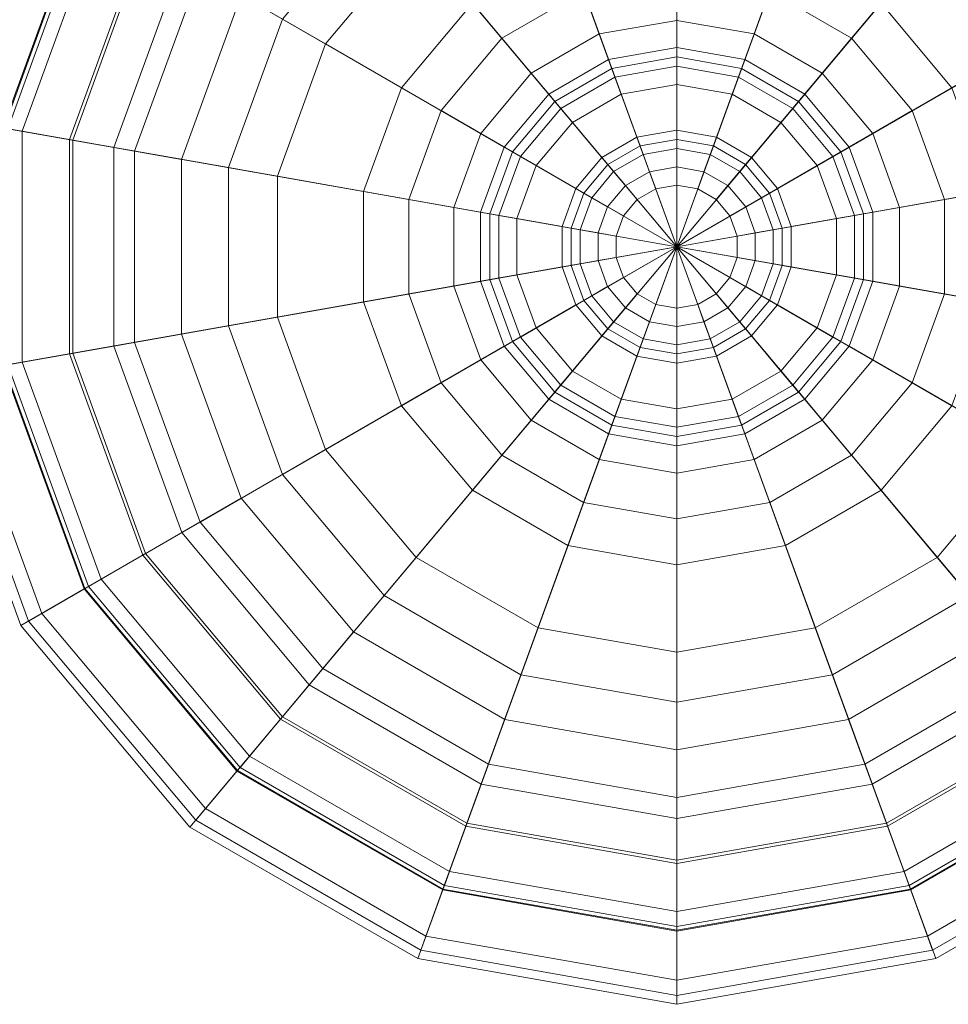
# Model space of a CAD drawing. Units: inches. Extents: x 375 to 1122, y 27 to 1069.
# Tile 48 of 155: x 720.906 to 722.566, y 309.111 to 310.871. Entities that reach past the tile are written whole.
import ezdxf

# ---------------------------------------------------------------- set-up
doc = ezdxf.new("R2010")
doc.units = ezdxf.units.IN
doc.layers.add('Furniture', color=30, linetype='Continuous', lineweight=18)

# ---------------------------------------------------------------- blocks, each defined once
blk = doc.blocks.new('A$C403C54AD')
for points in [[(0.889855, 0.961682, -0.042784), (0.895735, 0.928335, -0.039705), (0.895735, 0.928335, -0.039705), (0.878804, 0.95766, -0.042784)], [(0.901615, 0.961682, -0.042784), (0.895735, 0.928335, -0.039705), (0.895735, 0.928335, -0.039705), (0.889855, 0.961682, -0.042784)], [(0.912666, 0.95766, -0.042784), (0.895735, 0.928335, -0.039705), (0.895735, 0.928335, -0.039705), (0.901615, 0.961682, -0.042784)], [(0.878804, 0.95766, -0.042784), (0.895735, 0.928335, -0.039705), (0.895735, 0.928335, -0.039705), (0.869795, 0.950101, -0.042784)], [(0.921675, 0.950101, -0.042784), (0.895735, 0.928335, -0.039705), (0.895735, 0.928335, -0.039705), (0.912666, 0.95766, -0.042784)], [(0.888627, 0.940645, -0.036278), (0.880436, 0.954832, -0.039553), (0.872296, 0.948002, -0.039553), (0.884846, 0.937471, -0.036278)], [(0.906623, 0.937471, -0.036278), (0.919173, 0.948002, -0.039553), (0.911033, 0.954832, -0.039553), (0.902842, 0.940645, -0.036278)], [(0.869795, 0.950101, -0.042784), (0.895735, 0.928335, -0.039705), (0.895735, 0.928335, -0.039705), (0.863915, 0.939916, -0.042784)], [(0.927555, 0.939916, -0.042784), (0.895735, 0.928335, -0.039705), (0.895735, 0.928335, -0.039705), (0.921675, 0.950101, -0.042784)], [(0.924448, 0.938785, 0.1202), (0.92718, 0.93978, 0.106976), (0.921369, 0.949844, 0.106976), (0.919142, 0.947976, 0.1202)], [(0.924486, 0.938799, -0.039553), (0.927555, 0.939916, -0.042784), (0.921675, 0.950101, -0.042784), (0.919173, 0.948002, -0.039553)], [(0.92718, 0.93978, 0.106976), (0.926546, 0.939549, 0.078734), (0.920852, 0.949411, 0.078734), (0.921369, 0.949844, 0.106976)], [(0.886671, 0.944033, 0.05268), (0.883428, 0.94965, 0.062072), (0.87688, 0.944156, 0.062072), (0.881848, 0.939987, 0.05268)], [(0.909621, 0.939987, 0.05268), (0.914589, 0.944156, 0.062072), (0.908041, 0.94965, 0.062072), (0.904798, 0.944033, 0.05268)], [(0.926546, 0.939549, 0.078734), (0.921505, 0.937714, 0.060725), (0.916743, 0.945962, 0.060725), (0.920852, 0.949411, 0.078734)], [(0.8922, 0.948383, 0.050493), (0.893978, 0.9383, 0.043125), (0.890675, 0.937098, 0.043125), (0.885556, 0.945965, 0.050493)], [(0.89927, 0.948383, 0.050493), (0.897492, 0.9383, 0.043125), (0.893978, 0.9383, 0.043125), (0.8922, 0.948383, 0.050493)], [(0.905913, 0.945965, 0.050493), (0.900794, 0.937098, 0.043125), (0.897492, 0.9383, 0.043125), (0.89927, 0.948383, 0.050493)], [(0.909092, 0.933196, -0.036278), (0.924486, 0.938799, -0.039553), (0.919173, 0.948002, -0.039553), (0.906623, 0.937471, -0.036278)], [(0.919753, 0.937076, 0.129606), (0.924448, 0.938785, 0.1202), (0.919142, 0.947976, 0.1202), (0.915314, 0.944764, 0.129606)], [(0.924281, 0.938725, 0.106759), (0.921641, 0.937764, 0.119395), (0.916854, 0.946056, 0.119395), (0.919006, 0.947862, 0.106759)], [(0.923663, 0.9385, 0.079219), (0.924281, 0.938725, 0.106759), (0.919006, 0.947862, 0.106759), (0.918502, 0.947439, 0.079219)], [(0.918863, 0.936753, 0.062072), (0.923663, 0.9385, 0.079219), (0.918502, 0.947439, 0.079219), (0.914589, 0.944156, 0.062072)], [(0.885556, 0.945965, 0.050493), (0.890675, 0.937098, 0.043125), (0.887983, 0.934839, 0.043125), (0.88014, 0.94142, 0.050493)], [(0.894188, 0.937103, 0.046044), (0.892587, 0.946186, 0.05268), (0.886671, 0.944033, 0.05268), (0.891283, 0.936046, 0.046044)], [(0.897281, 0.937103, 0.046044), (0.898882, 0.946186, 0.05268), (0.892587, 0.946186, 0.05268), (0.894188, 0.937103, 0.046044)], [(0.900187, 0.936046, 0.046044), (0.904798, 0.944033, 0.05268), (0.898882, 0.946186, 0.05268), (0.897281, 0.937103, 0.046044)], [(0.911329, 0.94142, 0.050493), (0.903486, 0.934839, 0.043125), (0.900794, 0.937098, 0.043125), (0.905913, 0.945965, 0.050493)], [(0.921505, 0.937714, 0.060725), (0.914864, 0.935297, 0.050493), (0.911329, 0.94142, 0.050493), (0.916743, 0.945962, 0.060725)], [(0.921641, 0.937764, 0.119395), (0.91686, 0.936024, 0.129606), (0.912956, 0.942785, 0.129606), (0.916854, 0.946056, 0.119395)], [(0.91686, 0.936024, 0.129606), (0.919753, 0.937076, 0.129606), (0.915314, 0.944764, 0.129606), (0.912956, 0.942785, 0.129606)], [(0.912769, 0.934534, 0.05268), (0.918863, 0.936753, 0.062072), (0.914589, 0.944156, 0.062072), (0.909621, 0.939987, 0.05268)], [(0.891283, 0.936046, 0.046044), (0.886671, 0.944033, 0.05268), (0.881848, 0.939987, 0.05268), (0.888914, 0.934058, 0.046044)], [(0.902556, 0.934058, 0.046044), (0.909621, 0.939987, 0.05268), (0.904798, 0.944033, 0.05268), (0.900187, 0.936046, 0.046044)], [(0.893622, 0.940316, -0.033413), (0.893266, 0.942333, -0.036278), (0.888627, 0.940645, -0.036278), (0.889651, 0.938871, -0.033413)], [(0.897847, 0.940316, -0.033413), (0.898203, 0.942333, -0.036278), (0.893266, 0.942333, -0.036278), (0.893622, 0.940316, -0.033413)], [(0.901818, 0.938871, -0.033413), (0.902842, 0.940645, -0.036278), (0.898203, 0.942333, -0.036278), (0.897847, 0.940316, -0.033413)], [(0.88014, 0.94142, 0.050493), (0.887983, 0.934839, 0.043125), (0.886226, 0.931795, 0.043125), (0.876605, 0.935297, 0.050493)], [(0.914864, 0.935297, 0.050493), (0.905243, 0.931795, 0.043125), (0.903486, 0.934839, 0.043125), (0.911329, 0.94142, 0.050493)], [(0.889651, 0.938871, -0.033413), (0.888627, 0.940645, -0.036278), (0.884846, 0.937471, -0.036278), (0.886415, 0.936155, -0.033413)], [(0.905055, 0.936155, -0.033413), (0.906623, 0.937471, -0.036278), (0.902842, 0.940645, -0.036278), (0.901818, 0.938871, -0.033413)], [(0.894333, 0.936283, -0.031367), (0.893622, 0.940316, -0.033413), (0.889651, 0.938871, -0.033413), (0.891699, 0.935324, -0.031367)], [(0.897136, 0.936283, -0.031367), (0.897847, 0.940316, -0.033413), (0.893622, 0.940316, -0.033413), (0.894333, 0.936283, -0.031367)], [(0.89977, 0.935324, -0.031367), (0.901818, 0.938871, -0.033413), (0.897847, 0.940316, -0.033413), (0.897136, 0.936283, -0.031367)], [(0.863915, 0.939916, -0.042784), (0.895735, 0.928335, -0.039705), (0.895735, 0.928335, -0.039705), (0.861872, 0.928335, -0.042784)], [(0.888914, 0.934058, 0.046044), (0.881848, 0.939987, 0.05268), (0.878701, 0.934534, 0.05268), (0.887368, 0.93138, 0.046044)], [(0.929597, 0.928335, -0.042784), (0.895735, 0.928335, -0.039705), (0.895735, 0.928335, -0.039705), (0.927555, 0.939916, -0.042784)], [(0.904102, 0.93138, 0.046044), (0.912769, 0.934534, 0.05268), (0.909621, 0.939987, 0.05268), (0.902556, 0.934058, 0.046044)], [(0.926291, 0.928335, 0.1202), (0.929198, 0.928335, 0.106976), (0.92718, 0.93978, 0.106976), (0.924448, 0.938785, 0.1202)], [(0.926331, 0.928335, -0.039553), (0.929597, 0.928335, -0.042784), (0.927555, 0.939916, -0.042784), (0.924486, 0.938799, -0.039553)], [(0.929198, 0.928335, 0.106976), (0.928523, 0.928335, 0.078734), (0.926546, 0.939549, 0.078734), (0.92718, 0.93978, 0.106976)], [(0.928523, 0.928335, 0.078734), (0.923158, 0.928335, 0.060725), (0.921505, 0.937714, 0.060725), (0.926546, 0.939549, 0.078734)], [(0.891699, 0.935324, -0.031367), (0.889651, 0.938871, -0.033413), (0.886415, 0.936155, -0.033413), (0.889552, 0.933523, -0.031367)], [(0.901917, 0.933523, -0.031367), (0.905055, 0.936155, -0.033413), (0.901818, 0.938871, -0.033413), (0.89977, 0.935324, -0.031367)], [(0.909949, 0.928335, -0.036278), (0.926331, 0.928335, -0.039553), (0.924486, 0.938799, -0.039553), (0.909092, 0.933196, -0.036278)], [(0.921294, 0.928335, 0.129606), (0.926291, 0.928335, 0.1202), (0.924448, 0.938785, 0.1202), (0.919753, 0.937076, 0.129606)], [(0.920348, 0.928335, 0.062072), (0.925455, 0.928335, 0.079219), (0.923663, 0.9385, 0.079219), (0.918863, 0.936753, 0.062072)], [(0.926113, 0.928335, 0.106759), (0.923304, 0.928335, 0.119395), (0.921641, 0.937764, 0.119395), (0.924281, 0.938725, 0.106759)], [(0.925455, 0.928335, 0.079219), (0.926113, 0.928335, 0.106759), (0.924281, 0.938725, 0.106759), (0.923663, 0.9385, 0.079219)], [(0.893978, 0.9383, 0.043125), (0.894831, 0.93346, 0.042307), (0.893133, 0.932841, 0.042307), (0.890675, 0.937098, 0.043125)], [(0.897492, 0.9383, 0.043125), (0.896638, 0.93346, 0.042307), (0.894831, 0.93346, 0.042307), (0.893978, 0.9383, 0.043125)], [(0.900794, 0.937098, 0.043125), (0.898337, 0.932841, 0.042307), (0.896638, 0.93346, 0.042307), (0.897492, 0.9383, 0.043125)], [(0.886415, 0.936155, -0.033413), (0.884846, 0.937471, -0.036278), (0.882378, 0.933196, -0.036278), (0.884302, 0.932496, -0.033413)], [(0.907167, 0.932496, -0.033413), (0.909092, 0.933196, -0.036278), (0.906623, 0.937471, -0.036278), (0.905055, 0.936155, -0.033413)], [(0.923158, 0.928335, 0.060725), (0.916092, 0.928335, 0.050493), (0.914864, 0.935297, 0.050493), (0.921505, 0.937714, 0.060725)], [(0.923304, 0.928335, 0.119395), (0.918216, 0.928335, 0.129606), (0.91686, 0.936024, 0.129606), (0.921641, 0.937764, 0.119395)], [(0.890675, 0.937098, 0.043125), (0.893133, 0.932841, 0.042307), (0.891748, 0.93168, 0.042307), (0.887983, 0.934839, 0.043125)], [(0.895735, 0.928335, 0.044561), (0.894188, 0.937103, 0.046044), (0.891283, 0.936046, 0.046044), (0.895735, 0.928335, 0.044561)], [(0.895735, 0.928335, 0.044561), (0.897281, 0.937103, 0.046044), (0.894188, 0.937103, 0.046044), (0.895735, 0.928335, 0.044561)], [(0.895735, 0.928335, 0.044561), (0.900187, 0.936046, 0.046044), (0.897281, 0.937103, 0.046044), (0.895735, 0.928335, 0.044561)], [(0.903486, 0.934839, 0.043125), (0.899721, 0.93168, 0.042307), (0.898337, 0.932841, 0.042307), (0.900794, 0.937098, 0.043125)], [(0.918216, 0.928335, 0.129606), (0.921294, 0.928335, 0.129606), (0.919753, 0.937076, 0.129606), (0.91686, 0.936024, 0.129606)], [(0.894475, 0.935476, 0.041488), (0.894262, 0.936686, 0.039442), (0.891494, 0.935679, 0.039442), (0.892109, 0.934615, 0.041488)], [(0.894262, 0.936686, 0.039442), (0.894973, 0.932653, 0.037395), (0.893542, 0.932132, 0.037395), (0.891494, 0.935679, 0.039442)], [(0.896994, 0.935476, 0.041488), (0.897207, 0.936686, 0.039442), (0.894262, 0.936686, 0.039442), (0.894475, 0.935476, 0.041488)], [(0.897207, 0.936686, 0.039442), (0.896496, 0.932653, 0.037395), (0.894973, 0.932653, 0.037395), (0.894262, 0.936686, 0.039442)], [(0.899975, 0.935679, 0.039442), (0.897927, 0.932132, 0.037395), (0.896496, 0.932653, 0.037395), (0.897207, 0.936686, 0.039442)], [(0.899361, 0.934615, 0.041488), (0.899975, 0.935679, 0.039442), (0.897207, 0.936686, 0.039442), (0.896994, 0.935476, 0.041488)], [(0.913862, 0.928335, 0.05268), (0.920348, 0.928335, 0.062072), (0.918863, 0.936753, 0.062072), (0.912769, 0.934534, 0.05268)], [(0.889552, 0.933523, -0.031367), (0.886415, 0.936155, -0.033413), (0.884302, 0.932496, -0.033413), (0.88815, 0.931095, -0.031367)], [(0.894902, 0.933056, -0.026046), (0.894333, 0.936283, -0.031367), (0.891699, 0.935324, -0.031367), (0.893337, 0.932487, -0.026046)], [(0.896567, 0.933056, -0.026046), (0.897136, 0.936283, -0.031367), (0.894333, 0.936283, -0.031367), (0.894902, 0.933056, -0.026046)], [(0.898132, 0.932487, -0.026046), (0.89977, 0.935324, -0.031367), (0.897136, 0.936283, -0.031367), (0.896567, 0.933056, -0.026046)], [(0.903319, 0.931095, -0.031367), (0.907167, 0.932496, -0.033413), (0.905055, 0.936155, -0.033413), (0.901917, 0.933523, -0.031367)], [(0.895735, 0.928335, 0.044561), (0.891283, 0.936046, 0.046044), (0.888914, 0.934058, 0.046044), (0.895735, 0.928335, 0.044561)], [(0.891494, 0.935679, 0.039442), (0.893542, 0.932132, 0.037395), (0.892376, 0.931153, 0.037395), (0.889238, 0.933786, 0.039442)], [(0.892109, 0.934615, 0.041488), (0.891494, 0.935679, 0.039442), (0.889238, 0.933786, 0.039442), (0.890179, 0.932996, 0.041488)], [(0.895735, 0.928335, 0.044561), (0.902556, 0.934058, 0.046044), (0.900187, 0.936046, 0.046044), (0.895735, 0.928335, 0.044561)], [(0.902231, 0.933786, 0.039442), (0.899094, 0.931153, 0.037395), (0.897927, 0.932132, 0.037395), (0.899975, 0.935679, 0.039442)], [(0.90129, 0.932996, 0.041488), (0.902231, 0.933786, 0.039442), (0.899975, 0.935679, 0.039442), (0.899361, 0.934615, 0.041488)], [(0.876605, 0.935297, 0.050493), (0.886226, 0.931795, 0.043125), (0.885616, 0.928335, 0.043125), (0.875377, 0.928335, 0.050493)], [(0.893337, 0.932487, -0.026046), (0.891699, 0.935324, -0.031367), (0.889552, 0.933523, -0.031367), (0.892062, 0.931416, -0.026046)], [(0.894831, 0.93346, 0.042307), (0.894475, 0.935476, 0.041488), (0.892109, 0.934615, 0.041488), (0.893133, 0.932841, 0.042307)], [(0.896638, 0.93346, 0.042307), (0.896994, 0.935476, 0.041488), (0.894475, 0.935476, 0.041488), (0.894831, 0.93346, 0.042307)], [(0.898337, 0.932841, 0.042307), (0.899361, 0.934615, 0.041488), (0.896994, 0.935476, 0.041488), (0.896638, 0.93346, 0.042307)], [(0.899407, 0.931416, -0.026046), (0.901917, 0.933523, -0.031367), (0.89977, 0.935324, -0.031367), (0.898132, 0.932487, -0.026046)], [(0.916092, 0.928335, 0.050493), (0.905853, 0.928335, 0.043125), (0.905243, 0.931795, 0.043125), (0.914864, 0.935297, 0.050493)], [(0.887983, 0.934839, 0.043125), (0.891748, 0.93168, 0.042307), (0.890844, 0.930114, 0.042307), (0.886226, 0.931795, 0.043125)], [(0.905243, 0.931795, 0.043125), (0.900625, 0.930114, 0.042307), (0.899721, 0.93168, 0.042307), (0.903486, 0.934839, 0.043125)], [(0.887368, 0.93138, 0.046044), (0.878701, 0.934534, 0.05268), (0.877607, 0.928335, 0.05268), (0.886831, 0.928335, 0.046044)], [(0.893133, 0.932841, 0.042307), (0.892109, 0.934615, 0.041488), (0.890179, 0.932996, 0.041488), (0.891748, 0.93168, 0.042307)], [(0.899721, 0.93168, 0.042307), (0.90129, 0.932996, 0.041488), (0.899361, 0.934615, 0.041488), (0.898337, 0.932841, 0.042307)], [(0.904639, 0.928335, 0.046044), (0.913862, 0.928335, 0.05268), (0.912769, 0.934534, 0.05268), (0.904102, 0.93138, 0.046044)], [(0.895735, 0.928335, 0.044561), (0.888914, 0.934058, 0.046044), (0.887368, 0.93138, 0.046044), (0.895735, 0.928335, 0.044561)], [(0.895735, 0.928335, 0.044561), (0.904102, 0.93138, 0.046044), (0.902556, 0.934058, 0.046044), (0.895735, 0.928335, 0.044561)], [(0.889238, 0.933786, 0.039442), (0.892376, 0.931153, 0.037395), (0.891614, 0.929834, 0.037395), (0.887766, 0.931235, 0.039442)], [(0.890179, 0.932996, 0.041488), (0.889238, 0.933786, 0.039442), (0.887766, 0.931235, 0.039442), (0.88892, 0.930815, 0.041488)], [(0.892062, 0.931416, -0.026046), (0.889552, 0.933523, -0.031367), (0.88815, 0.931095, -0.031367), (0.891229, 0.929974, -0.026046)], [(0.903704, 0.931235, 0.039442), (0.899855, 0.929834, 0.037395), (0.899094, 0.931153, 0.037395), (0.902231, 0.933786, 0.039442)], [(0.90024, 0.929974, -0.026046), (0.903319, 0.931095, -0.031367), (0.901917, 0.933523, -0.031367), (0.899407, 0.931416, -0.026046)], [(0.902549, 0.930815, 0.041488), (0.903704, 0.931235, 0.039442), (0.902231, 0.933786, 0.039442), (0.90129, 0.932996, 0.041488)], [(0.895115, 0.931846, -0.017451), (0.894902, 0.933056, -0.026046), (0.893337, 0.932487, -0.026046), (0.893952, 0.931423, -0.017451)], [(0.896354, 0.931846, -0.017451), (0.896567, 0.933056, -0.026046), (0.894902, 0.933056, -0.026046), (0.895115, 0.931846, -0.017451)], [(0.897518, 0.931423, -0.017451), (0.898132, 0.932487, -0.026046), (0.896567, 0.933056, -0.026046), (0.896354, 0.931846, -0.017451)], [(0.907901, 0.928335, -0.033413), (0.909949, 0.928335, -0.036278), (0.909092, 0.933196, -0.036278), (0.907167, 0.932496, -0.033413)], [(0.891748, 0.93168, 0.042307), (0.890179, 0.932996, 0.041488), (0.88892, 0.930815, 0.041488), (0.890844, 0.930114, 0.042307)], [(0.894973, 0.932653, 0.037395), (0.895258, 0.93104, 0.030847), (0.894361, 0.930713, 0.030847), (0.893542, 0.932132, 0.037395)], [(0.896496, 0.932653, 0.037395), (0.896212, 0.93104, 0.030847), (0.895258, 0.93104, 0.030847), (0.894973, 0.932653, 0.037395)], [(0.897927, 0.932132, 0.037395), (0.897108, 0.930713, 0.030847), (0.896212, 0.93104, 0.030847), (0.896496, 0.932653, 0.037395)], [(0.900625, 0.930114, 0.042307), (0.902549, 0.930815, 0.041488), (0.90129, 0.932996, 0.041488), (0.899721, 0.93168, 0.042307)], [(0.88815, 0.931095, -0.031367), (0.884302, 0.932496, -0.033413), (0.883568, 0.928335, -0.033413), (0.887664, 0.928335, -0.031367)], [(0.893952, 0.931423, -0.017451), (0.893337, 0.932487, -0.026046), (0.892062, 0.931416, -0.026046), (0.893003, 0.930627, -0.017451)], [(0.898466, 0.930627, -0.017451), (0.899407, 0.931416, -0.026046), (0.898132, 0.932487, -0.026046), (0.897518, 0.931423, -0.017451)], [(0.903806, 0.928335, -0.031367), (0.907901, 0.928335, -0.033413), (0.907167, 0.932496, -0.033413), (0.903319, 0.931095, -0.031367)], [(0.886226, 0.931795, 0.043125), (0.890844, 0.930114, 0.042307), (0.890531, 0.928335, 0.042307), (0.885616, 0.928335, 0.043125)], [(0.893542, 0.932132, 0.037395), (0.894361, 0.930713, 0.030847), (0.89363, 0.9301, 0.030847), (0.892376, 0.931153, 0.037395)], [(0.895258, 0.93104, 0.030847), (0.895115, 0.931846, -0.017451), (0.893952, 0.931423, -0.017451), (0.894361, 0.930713, 0.030847)], [(0.896212, 0.93104, 0.030847), (0.896354, 0.931846, -0.017451), (0.895115, 0.931846, -0.017451), (0.895258, 0.93104, 0.030847)], [(0.897108, 0.930713, 0.030847), (0.897518, 0.931423, -0.017451), (0.896354, 0.931846, -0.017451), (0.896212, 0.93104, 0.030847)], [(0.899094, 0.931153, 0.037395), (0.897839, 0.9301, 0.030847), (0.897108, 0.930713, 0.030847), (0.897927, 0.932132, 0.037395)], [(0.905853, 0.928335, 0.043125), (0.900939, 0.928335, 0.042307), (0.900625, 0.930114, 0.042307), (0.905243, 0.931795, 0.043125)], [(0.895735, 0.928335, 0.044561), (0.887368, 0.93138, 0.046044), (0.886831, 0.928335, 0.046044), (0.895735, 0.928335, 0.044561)], [(0.893003, 0.930627, -0.017451), (0.892062, 0.931416, -0.026046), (0.891229, 0.929974, -0.026046), (0.892384, 0.929554, -0.017451)], [(0.894361, 0.930713, 0.030847), (0.893952, 0.931423, -0.017451), (0.893003, 0.930627, -0.017451), (0.89363, 0.9301, 0.030847)], [(0.895735, 0.928335, 0.044561), (0.904639, 0.928335, 0.046044), (0.904102, 0.93138, 0.046044), (0.895735, 0.928335, 0.044561)], [(0.897839, 0.9301, 0.030847), (0.898466, 0.930627, -0.017451), (0.897518, 0.931423, -0.017451), (0.897108, 0.930713, 0.030847)], [(0.899085, 0.929554, -0.017451), (0.90024, 0.929974, -0.026046), (0.899407, 0.931416, -0.026046), (0.898466, 0.930627, -0.017451)], [(0.887766, 0.931235, 0.039442), (0.891614, 0.929834, 0.037395), (0.89135, 0.928335, 0.037395), (0.887254, 0.928335, 0.039442)], [(0.88892, 0.930815, 0.041488), (0.887766, 0.931235, 0.039442), (0.887254, 0.928335, 0.039442), (0.888483, 0.928335, 0.041488)], [(0.891229, 0.929974, -0.026046), (0.88815, 0.931095, -0.031367), (0.887664, 0.928335, -0.031367), (0.89094, 0.928335, -0.026046)], [(0.892376, 0.931153, 0.037395), (0.89363, 0.9301, 0.030847), (0.893153, 0.929274, 0.030847), (0.891614, 0.929834, 0.037395)], [(0.899855, 0.929834, 0.037395), (0.898316, 0.929274, 0.030847), (0.897839, 0.9301, 0.030847), (0.899094, 0.931153, 0.037395)], [(0.904215, 0.928335, 0.039442), (0.90012, 0.928335, 0.037395), (0.899855, 0.929834, 0.037395), (0.903704, 0.931235, 0.039442)], [(0.900529, 0.928335, -0.026046), (0.903806, 0.928335, -0.031367), (0.903319, 0.931095, -0.031367), (0.90024, 0.929974, -0.026046)], [(0.902987, 0.928335, 0.041488), (0.904215, 0.928335, 0.039442), (0.903704, 0.931235, 0.039442), (0.902549, 0.930815, 0.041488)], [(0.890844, 0.930114, 0.042307), (0.88892, 0.930815, 0.041488), (0.888483, 0.928335, 0.041488), (0.890531, 0.928335, 0.042307)], [(0.89363, 0.9301, 0.030847), (0.893003, 0.930627, -0.017451), (0.892384, 0.929554, -0.017451), (0.893153, 0.929274, 0.030847)], [(0.898316, 0.929274, 0.030847), (0.899085, 0.929554, -0.017451), (0.898466, 0.930627, -0.017451), (0.897839, 0.9301, 0.030847)], [(0.900939, 0.928335, 0.042307), (0.902987, 0.928335, 0.041488), (0.902549, 0.930815, 0.041488), (0.900625, 0.930114, 0.042307)], [(0.892384, 0.929554, -0.017451), (0.891229, 0.929974, -0.026046), (0.89094, 0.928335, -0.026046), (0.892169, 0.928335, -0.017451)], [(0.899301, 0.928335, -0.017451), (0.900529, 0.928335, -0.026046), (0.90024, 0.929974, -0.026046), (0.899085, 0.929554, -0.017451)], [(0.891614, 0.929834, 0.037395), (0.893153, 0.929274, 0.030847), (0.892988, 0.928335, 0.030847), (0.89135, 0.928335, 0.037395)], [(0.893153, 0.929274, 0.030847), (0.892384, 0.929554, -0.017451), (0.892169, 0.928335, -0.017451), (0.892988, 0.928335, 0.030847)], [(0.90012, 0.928335, 0.037395), (0.898481, 0.928335, 0.030847), (0.898316, 0.929274, 0.030847), (0.899855, 0.929834, 0.037395)], [(0.898481, 0.928335, 0.030847), (0.899301, 0.928335, -0.017451), (0.899085, 0.929554, -0.017451), (0.898316, 0.929274, 0.030847)], [(0.861872, 0.928335, -0.042784), (0.895735, 0.928335, -0.039705), (0.895735, 0.928335, -0.039705), (0.863915, 0.916753, -0.042784)], [(0.863915, 0.916753, -0.042784), (0.895735, 0.928335, -0.039705), (0.895735, 0.928335, -0.039705), (0.869795, 0.906568, -0.042784)], [(0.869795, 0.906568, -0.042784), (0.895735, 0.928335, -0.039705), (0.895735, 0.928335, -0.039705), (0.878804, 0.899009, -0.042784)], [(0.875377, 0.928335, 0.050493), (0.885616, 0.928335, 0.043125), (0.886226, 0.924874, 0.043125), (0.876605, 0.921372, 0.050493)], [(0.886831, 0.928335, 0.046044), (0.877607, 0.928335, 0.05268), (0.878701, 0.922135, 0.05268), (0.887368, 0.925289, 0.046044)], [(0.878804, 0.899009, -0.042784), (0.895735, 0.928335, -0.039705), (0.895735, 0.928335, -0.039705), (0.889855, 0.894987, -0.042784)], [(0.887664, 0.928335, -0.031367), (0.883568, 0.928335, -0.033413), (0.884302, 0.924173, -0.033413), (0.88815, 0.925574, -0.031367)], [(0.885616, 0.928335, 0.043125), (0.890531, 0.928335, 0.042307), (0.890844, 0.926555, 0.042307), (0.886226, 0.924874, 0.043125)], [(0.895735, 0.928335, 0.044561), (0.886831, 0.928335, 0.046044), (0.887368, 0.925289, 0.046044), (0.895735, 0.928335, 0.044561)], [(0.887254, 0.928335, 0.039442), (0.89135, 0.928335, 0.037395), (0.891614, 0.926835, 0.037395), (0.887766, 0.925434, 0.039442)], [(0.888483, 0.928335, 0.041488), (0.887254, 0.928335, 0.039442), (0.887766, 0.925434, 0.039442), (0.88892, 0.925854, 0.041488)], [(0.895735, 0.928335, 0.044561), (0.887368, 0.925289, 0.046044), (0.888914, 0.922611, 0.046044), (0.895735, 0.928335, 0.044561)], [(0.89094, 0.928335, -0.026046), (0.887664, 0.928335, -0.031367), (0.88815, 0.925574, -0.031367), (0.891229, 0.926695, -0.026046)], [(0.890531, 0.928335, 0.042307), (0.888483, 0.928335, 0.041488), (0.88892, 0.925854, 0.041488), (0.890844, 0.926555, 0.042307)], [(0.895735, 0.928335, 0.044561), (0.888914, 0.922611, 0.046044), (0.891283, 0.920623, 0.046044), (0.895735, 0.928335, 0.044561)], [(0.889855, 0.894987, -0.042784), (0.895735, 0.928335, -0.039705), (0.895735, 0.928335, -0.039705), (0.901615, 0.894987, -0.042784)], [(0.892169, 0.928335, -0.017451), (0.89094, 0.928335, -0.026046), (0.891229, 0.926695, -0.026046), (0.892384, 0.927115, -0.017451)], [(0.895735, 0.928335, 0.044561), (0.891283, 0.920623, 0.046044), (0.894188, 0.919566, 0.046044), (0.895735, 0.928335, 0.044561)], [(0.89135, 0.928335, 0.037395), (0.892988, 0.928335, 0.030847), (0.893153, 0.927395, 0.030847), (0.891614, 0.926835, 0.037395)], [(0.892988, 0.928335, 0.030847), (0.892169, 0.928335, -0.017451), (0.892384, 0.927115, -0.017451), (0.893153, 0.927395, 0.030847)], [(0.895735, 0.928335, 0.044561), (0.894188, 0.919566, 0.046044), (0.897281, 0.919566, 0.046044), (0.895735, 0.928335, 0.044561)], [(0.895735, 0.928335, 0.044561), (0.904102, 0.925289, 0.046044), (0.904639, 0.928335, 0.046044), (0.895735, 0.928335, 0.044561)], [(0.895735, 0.928335, 0.044561), (0.902556, 0.922611, 0.046044), (0.904102, 0.925289, 0.046044), (0.895735, 0.928335, 0.044561)], [(0.895735, 0.928335, 0.044561), (0.900187, 0.920623, 0.046044), (0.902556, 0.922611, 0.046044), (0.895735, 0.928335, 0.044561)], [(0.895735, 0.928335, 0.044561), (0.897281, 0.919566, 0.046044), (0.900187, 0.920623, 0.046044), (0.895735, 0.928335, 0.044561)], [(0.927555, 0.916753, -0.042784), (0.895735, 0.928335, -0.039705), (0.895735, 0.928335, -0.039705), (0.929597, 0.928335, -0.042784)], [(0.921675, 0.906568, -0.042784), (0.895735, 0.928335, -0.039705), (0.895735, 0.928335, -0.039705), (0.927555, 0.916753, -0.042784)], [(0.912666, 0.899009, -0.042784), (0.895735, 0.928335, -0.039705), (0.895735, 0.928335, -0.039705), (0.921675, 0.906568, -0.042784)], [(0.901615, 0.894987, -0.042784), (0.895735, 0.928335, -0.039705), (0.895735, 0.928335, -0.039705), (0.912666, 0.899009, -0.042784)], [(0.899855, 0.926835, 0.037395), (0.898316, 0.927395, 0.030847), (0.898481, 0.928335, 0.030847), (0.90012, 0.928335, 0.037395)], [(0.898316, 0.927395, 0.030847), (0.899085, 0.927115, -0.017451), (0.899301, 0.928335, -0.017451), (0.898481, 0.928335, 0.030847)], [(0.899085, 0.927115, -0.017451), (0.90024, 0.926695, -0.026046), (0.900529, 0.928335, -0.026046), (0.899301, 0.928335, -0.017451)], [(0.903704, 0.925434, 0.039442), (0.899855, 0.926835, 0.037395), (0.90012, 0.928335, 0.037395), (0.904215, 0.928335, 0.039442)], [(0.90024, 0.926695, -0.026046), (0.903319, 0.925574, -0.031367), (0.903806, 0.928335, -0.031367), (0.900529, 0.928335, -0.026046)], [(0.900625, 0.926555, 0.042307), (0.902549, 0.925854, 0.041488), (0.902987, 0.928335, 0.041488), (0.900939, 0.928335, 0.042307)], [(0.905243, 0.924874, 0.043125), (0.900625, 0.926555, 0.042307), (0.900939, 0.928335, 0.042307), (0.905853, 0.928335, 0.043125)], [(0.902549, 0.925854, 0.041488), (0.903704, 0.925434, 0.039442), (0.904215, 0.928335, 0.039442), (0.902987, 0.928335, 0.041488)], [(0.903319, 0.925574, -0.031367), (0.907167, 0.924173, -0.033413), (0.907901, 0.928335, -0.033413), (0.903806, 0.928335, -0.031367)], [(0.904102, 0.925289, 0.046044), (0.912769, 0.922135, 0.05268), (0.913862, 0.928335, 0.05268), (0.904639, 0.928335, 0.046044)], [(0.914864, 0.921372, 0.050493), (0.905243, 0.924874, 0.043125), (0.905853, 0.928335, 0.043125), (0.916092, 0.928335, 0.050493)], [(0.907167, 0.924173, -0.033413), (0.909092, 0.923473, -0.036278), (0.909949, 0.928335, -0.036278), (0.907901, 0.928335, -0.033413)], [(0.909092, 0.923473, -0.036278), (0.924486, 0.91787, -0.039553), (0.926331, 0.928335, -0.039553), (0.909949, 0.928335, -0.036278)], [(0.912769, 0.922135, 0.05268), (0.918863, 0.919916, 0.062072), (0.920348, 0.928335, 0.062072), (0.913862, 0.928335, 0.05268)], [(0.921505, 0.918955, 0.060725), (0.914864, 0.921372, 0.050493), (0.916092, 0.928335, 0.050493), (0.923158, 0.928335, 0.060725)], [(0.91686, 0.920646, 0.129606), (0.919753, 0.919593, 0.129606), (0.921294, 0.928335, 0.129606), (0.918216, 0.928335, 0.129606)], [(0.921641, 0.918905, 0.119395), (0.91686, 0.920646, 0.129606), (0.918216, 0.928335, 0.129606), (0.923304, 0.928335, 0.119395)], [(0.918863, 0.919916, 0.062072), (0.923663, 0.918169, 0.079219), (0.925455, 0.928335, 0.079219), (0.920348, 0.928335, 0.062072)], [(0.919753, 0.919593, 0.129606), (0.924448, 0.917884, 0.1202), (0.926291, 0.928335, 0.1202), (0.921294, 0.928335, 0.129606)], [(0.926546, 0.91712, 0.078734), (0.921505, 0.918955, 0.060725), (0.923158, 0.928335, 0.060725), (0.928523, 0.928335, 0.078734)], [(0.924281, 0.917944, 0.106759), (0.921641, 0.918905, 0.119395), (0.923304, 0.928335, 0.119395), (0.926113, 0.928335, 0.106759)], [(0.923663, 0.918169, 0.079219), (0.924281, 0.917944, 0.106759), (0.926113, 0.928335, 0.106759), (0.925455, 0.928335, 0.079219)], [(0.924448, 0.917884, 0.1202), (0.92718, 0.916889, 0.106976), (0.929198, 0.928335, 0.106976), (0.926291, 0.928335, 0.1202)], [(0.924486, 0.91787, -0.039553), (0.927555, 0.916753, -0.042784), (0.929597, 0.928335, -0.042784), (0.926331, 0.928335, -0.039553)], [(0.92718, 0.916889, 0.106976), (0.926546, 0.91712, 0.078734), (0.928523, 0.928335, 0.078734), (0.929198, 0.928335, 0.106976)], [(0.891614, 0.926835, 0.037395), (0.893153, 0.927395, 0.030847), (0.89363, 0.926569, 0.030847), (0.892376, 0.925516, 0.037395)], [(0.893153, 0.927395, 0.030847), (0.892384, 0.927115, -0.017451), (0.893003, 0.926042, -0.017451), (0.89363, 0.926569, 0.030847)], [(0.899094, 0.925516, 0.037395), (0.897839, 0.926569, 0.030847), (0.898316, 0.927395, 0.030847), (0.899855, 0.926835, 0.037395)], [(0.897839, 0.926569, 0.030847), (0.898466, 0.926042, -0.017451), (0.899085, 0.927115, -0.017451), (0.898316, 0.927395, 0.030847)], [(0.892384, 0.927115, -0.017451), (0.891229, 0.926695, -0.026046), (0.892062, 0.925253, -0.026046), (0.893003, 0.926042, -0.017451)], [(0.898466, 0.926042, -0.017451), (0.899407, 0.925253, -0.026046), (0.90024, 0.926695, -0.026046), (0.899085, 0.927115, -0.017451)], [(0.886226, 0.924874, 0.043125), (0.890844, 0.926555, 0.042307), (0.891748, 0.924989, 0.042307), (0.887983, 0.92183, 0.043125)], [(0.887766, 0.925434, 0.039442), (0.891614, 0.926835, 0.037395), (0.892376, 0.925516, 0.037395), (0.889238, 0.922883, 0.039442)], [(0.891229, 0.926695, -0.026046), (0.88815, 0.925574, -0.031367), (0.889552, 0.923147, -0.031367), (0.892062, 0.925253, -0.026046)], [(0.890844, 0.926555, 0.042307), (0.88892, 0.925854, 0.041488), (0.890179, 0.923673, 0.041488), (0.891748, 0.924989, 0.042307)], [(0.892376, 0.925516, 0.037395), (0.89363, 0.926569, 0.030847), (0.894361, 0.925956, 0.030847), (0.893542, 0.924537, 0.037395)], [(0.89363, 0.926569, 0.030847), (0.893003, 0.926042, -0.017451), (0.893952, 0.925246, -0.017451), (0.894361, 0.925956, 0.030847)], [(0.897927, 0.924537, 0.037395), (0.897108, 0.925956, 0.030847), (0.897839, 0.926569, 0.030847), (0.899094, 0.925516, 0.037395)], [(0.897108, 0.925956, 0.030847), (0.897518, 0.925246, -0.017451), (0.898466, 0.926042, -0.017451), (0.897839, 0.926569, 0.030847)], [(0.902231, 0.922883, 0.039442), (0.899094, 0.925516, 0.037395), (0.899855, 0.926835, 0.037395), (0.903704, 0.925434, 0.039442)], [(0.899407, 0.925253, -0.026046), (0.901917, 0.923147, -0.031367), (0.903319, 0.925574, -0.031367), (0.90024, 0.926695, -0.026046)], [(0.899721, 0.924989, 0.042307), (0.90129, 0.923673, 0.041488), (0.902549, 0.925854, 0.041488), (0.900625, 0.926555, 0.042307)], [(0.903486, 0.92183, 0.043125), (0.899721, 0.924989, 0.042307), (0.900625, 0.926555, 0.042307), (0.905243, 0.924874, 0.043125)], [(0.893003, 0.926042, -0.017451), (0.892062, 0.925253, -0.026046), (0.893337, 0.924182, -0.026046), (0.893952, 0.925246, -0.017451)], [(0.897518, 0.925246, -0.017451), (0.898132, 0.924182, -0.026046), (0.899407, 0.925253, -0.026046), (0.898466, 0.926042, -0.017451)], [(0.88815, 0.925574, -0.031367), (0.884302, 0.924173, -0.033413), (0.886415, 0.920514, -0.033413), (0.889552, 0.923147, -0.031367)], [(0.88892, 0.925854, 0.041488), (0.887766, 0.925434, 0.039442), (0.889238, 0.922883, 0.039442), (0.890179, 0.923673, 0.041488)], [(0.893542, 0.924537, 0.037395), (0.894361, 0.925956, 0.030847), (0.895258, 0.92563, 0.030847), (0.894973, 0.924016, 0.037395)], [(0.894361, 0.925956, 0.030847), (0.893952, 0.925246, -0.017451), (0.895115, 0.924823, -0.017451), (0.895258, 0.92563, 0.030847)], [(0.894973, 0.924016, 0.037395), (0.895258, 0.92563, 0.030847), (0.896212, 0.92563, 0.030847), (0.896496, 0.924016, 0.037395)], [(0.895258, 0.92563, 0.030847), (0.895115, 0.924823, -0.017451), (0.896354, 0.924823, -0.017451), (0.896212, 0.92563, 0.030847)], [(0.896496, 0.924016, 0.037395), (0.896212, 0.92563, 0.030847), (0.897108, 0.925956, 0.030847), (0.897927, 0.924537, 0.037395)], [(0.896212, 0.92563, 0.030847), (0.896354, 0.924823, -0.017451), (0.897518, 0.925246, -0.017451), (0.897108, 0.925956, 0.030847)], [(0.90129, 0.923673, 0.041488), (0.902231, 0.922883, 0.039442), (0.903704, 0.925434, 0.039442), (0.902549, 0.925854, 0.041488)], [(0.901917, 0.923147, -0.031367), (0.905055, 0.920514, -0.033413), (0.907167, 0.924173, -0.033413), (0.903319, 0.925574, -0.031367)], [(0.887368, 0.925289, 0.046044), (0.878701, 0.922135, 0.05268), (0.881848, 0.916683, 0.05268), (0.888914, 0.922611, 0.046044)], [(0.889238, 0.922883, 0.039442), (0.892376, 0.925516, 0.037395), (0.893542, 0.924537, 0.037395), (0.891494, 0.92099, 0.039442)], [(0.892062, 0.925253, -0.026046), (0.889552, 0.923147, -0.031367), (0.891699, 0.921345, -0.031367), (0.893337, 0.924182, -0.026046)], [(0.893952, 0.925246, -0.017451), (0.893337, 0.924182, -0.026046), (0.894902, 0.923613, -0.026046), (0.895115, 0.924823, -0.017451)], [(0.896354, 0.924823, -0.017451), (0.896567, 0.923613, -0.026046), (0.898132, 0.924182, -0.026046), (0.897518, 0.925246, -0.017451)], [(0.899975, 0.92099, 0.039442), (0.897927, 0.924537, 0.037395), (0.899094, 0.925516, 0.037395), (0.902231, 0.922883, 0.039442)], [(0.898132, 0.924182, -0.026046), (0.89977, 0.921345, -0.031367), (0.901917, 0.923147, -0.031367), (0.899407, 0.925253, -0.026046)], [(0.902556, 0.922611, 0.046044), (0.909621, 0.916683, 0.05268), (0.912769, 0.922135, 0.05268), (0.904102, 0.925289, 0.046044)], [(0.876605, 0.921372, 0.050493), (0.886226, 0.924874, 0.043125), (0.887983, 0.92183, 0.043125), (0.88014, 0.915249, 0.050493)], [(0.887983, 0.92183, 0.043125), (0.891748, 0.924989, 0.042307), (0.893133, 0.923828, 0.042307), (0.890675, 0.919571, 0.043125)], [(0.891748, 0.924989, 0.042307), (0.890179, 0.923673, 0.041488), (0.892109, 0.922054, 0.041488), (0.893133, 0.923828, 0.042307)], [(0.895115, 0.924823, -0.017451), (0.894902, 0.923613, -0.026046), (0.896567, 0.923613, -0.026046), (0.896354, 0.924823, -0.017451)], [(0.898337, 0.923828, 0.042307), (0.899361, 0.922054, 0.041488), (0.90129, 0.923673, 0.041488), (0.899721, 0.924989, 0.042307)], [(0.900794, 0.919571, 0.043125), (0.898337, 0.923828, 0.042307), (0.899721, 0.924989, 0.042307), (0.903486, 0.92183, 0.043125)], [(0.911329, 0.915249, 0.050493), (0.903486, 0.92183, 0.043125), (0.905243, 0.924874, 0.043125), (0.914864, 0.921372, 0.050493)], [(0.891494, 0.92099, 0.039442), (0.893542, 0.924537, 0.037395), (0.894973, 0.924016, 0.037395), (0.894262, 0.919983, 0.039442)], [(0.897207, 0.919983, 0.039442), (0.896496, 0.924016, 0.037395), (0.897927, 0.924537, 0.037395), (0.899975, 0.92099, 0.039442)], [(0.884302, 0.924173, -0.033413), (0.882378, 0.923473, -0.036278), (0.884846, 0.919198, -0.036278), (0.886415, 0.920514, -0.033413)], [(0.890675, 0.919571, 0.043125), (0.893133, 0.923828, 0.042307), (0.894831, 0.92321, 0.042307), (0.893978, 0.91837, 0.043125)], [(0.893337, 0.924182, -0.026046), (0.891699, 0.921345, -0.031367), (0.894333, 0.920386, -0.031367), (0.894902, 0.923613, -0.026046)], [(0.893133, 0.923828, 0.042307), (0.892109, 0.922054, 0.041488), (0.894475, 0.921193, 0.041488), (0.894831, 0.92321, 0.042307)], [(0.894262, 0.919983, 0.039442), (0.894973, 0.924016, 0.037395), (0.896496, 0.924016, 0.037395), (0.897207, 0.919983, 0.039442)], [(0.896567, 0.923613, -0.026046), (0.897136, 0.920386, -0.031367), (0.89977, 0.921345, -0.031367), (0.898132, 0.924182, -0.026046)], [(0.896638, 0.92321, 0.042307), (0.896994, 0.921193, 0.041488), (0.899361, 0.922054, 0.041488), (0.898337, 0.923828, 0.042307)], [(0.897492, 0.91837, 0.043125), (0.896638, 0.92321, 0.042307), (0.898337, 0.923828, 0.042307), (0.900794, 0.919571, 0.043125)], [(0.905055, 0.920514, -0.033413), (0.906623, 0.919198, -0.036278), (0.909092, 0.923473, -0.036278), (0.907167, 0.924173, -0.033413)], [(0.890179, 0.923673, 0.041488), (0.889238, 0.922883, 0.039442), (0.891494, 0.92099, 0.039442), (0.892109, 0.922054, 0.041488)], [(0.894902, 0.923613, -0.026046), (0.894333, 0.920386, -0.031367), (0.897136, 0.920386, -0.031367), (0.896567, 0.923613, -0.026046)], [(0.899361, 0.922054, 0.041488), (0.899975, 0.92099, 0.039442), (0.902231, 0.922883, 0.039442), (0.90129, 0.923673, 0.041488)], [(0.906623, 0.919198, -0.036278), (0.919173, 0.908668, -0.039553), (0.924486, 0.91787, -0.039553), (0.909092, 0.923473, -0.036278)], [(0.889552, 0.923147, -0.031367), (0.886415, 0.920514, -0.033413), (0.889651, 0.917798, -0.033413), (0.891699, 0.921345, -0.031367)], [(0.893978, 0.91837, 0.043125), (0.894831, 0.92321, 0.042307), (0.896638, 0.92321, 0.042307), (0.897492, 0.91837, 0.043125)], [(0.894831, 0.92321, 0.042307), (0.894475, 0.921193, 0.041488), (0.896994, 0.921193, 0.041488), (0.896638, 0.92321, 0.042307)], [(0.89977, 0.921345, -0.031367), (0.901818, 0.917798, -0.033413), (0.905055, 0.920514, -0.033413), (0.901917, 0.923147, -0.031367)], [(0.888914, 0.922611, 0.046044), (0.881848, 0.916683, 0.05268), (0.886671, 0.912636, 0.05268), (0.891283, 0.920623, 0.046044)], [(0.900187, 0.920623, 0.046044), (0.904798, 0.912636, 0.05268), (0.909621, 0.916683, 0.05268), (0.902556, 0.922611, 0.046044)], [(0.892109, 0.922054, 0.041488), (0.891494, 0.92099, 0.039442), (0.894262, 0.919983, 0.039442), (0.894475, 0.921193, 0.041488)], [(0.896994, 0.921193, 0.041488), (0.897207, 0.919983, 0.039442), (0.899975, 0.92099, 0.039442), (0.899361, 0.922054, 0.041488)], [(0.909621, 0.916683, 0.05268), (0.914589, 0.912514, 0.062072), (0.918863, 0.919916, 0.062072), (0.912769, 0.922135, 0.05268)], [(0.88014, 0.915249, 0.050493), (0.887983, 0.92183, 0.043125), (0.890675, 0.919571, 0.043125), (0.885556, 0.910704, 0.050493)], [(0.905913, 0.910704, 0.050493), (0.900794, 0.919571, 0.043125), (0.903486, 0.92183, 0.043125), (0.911329, 0.915249, 0.050493)], [(0.891699, 0.921345, -0.031367), (0.889651, 0.917798, -0.033413), (0.893622, 0.916353, -0.033413), (0.894333, 0.920386, -0.031367)], [(0.894475, 0.921193, 0.041488), (0.894262, 0.919983, 0.039442), (0.897207, 0.919983, 0.039442), (0.896994, 0.921193, 0.041488)], [(0.897136, 0.920386, -0.031367), (0.897847, 0.916353, -0.033413), (0.901818, 0.917798, -0.033413), (0.89977, 0.921345, -0.031367)], [(0.916743, 0.910707, 0.060725), (0.911329, 0.915249, 0.050493), (0.914864, 0.921372, 0.050493), (0.921505, 0.918955, 0.060725)], [(0.886415, 0.920514, -0.033413), (0.884846, 0.919198, -0.036278), (0.888627, 0.916025, -0.036278), (0.889651, 0.917798, -0.033413)], [(0.891283, 0.920623, 0.046044), (0.886671, 0.912636, 0.05268), (0.892587, 0.910483, 0.05268), (0.894188, 0.919566, 0.046044)], [(0.894333, 0.920386, -0.031367), (0.893622, 0.916353, -0.033413), (0.897847, 0.916353, -0.033413), (0.897136, 0.920386, -0.031367)], [(0.897281, 0.919566, 0.046044), (0.898882, 0.910483, 0.05268), (0.904798, 0.912636, 0.05268), (0.900187, 0.920623, 0.046044)], [(0.901818, 0.917798, -0.033413), (0.902842, 0.916025, -0.036278), (0.906623, 0.919198, -0.036278), (0.905055, 0.920514, -0.033413)], [(0.912956, 0.913884, 0.129606), (0.915314, 0.911905, 0.129606), (0.919753, 0.919593, 0.129606), (0.91686, 0.920646, 0.129606)], [(0.916854, 0.910614, 0.119395), (0.912956, 0.913884, 0.129606), (0.91686, 0.920646, 0.129606), (0.921641, 0.918905, 0.119395)], [(0.914589, 0.912514, 0.062072), (0.918502, 0.90923, 0.079219), (0.923663, 0.918169, 0.079219), (0.918863, 0.919916, 0.062072)], [(0.885556, 0.910704, 0.050493), (0.890675, 0.919571, 0.043125), (0.893978, 0.91837, 0.043125), (0.8922, 0.908286, 0.050493)], [(0.894188, 0.919566, 0.046044), (0.892587, 0.910483, 0.05268), (0.898882, 0.910483, 0.05268), (0.897281, 0.919566, 0.046044)], [(0.89927, 0.908286, 0.050493), (0.897492, 0.91837, 0.043125), (0.900794, 0.919571, 0.043125), (0.905913, 0.910704, 0.050493)], [(0.915314, 0.911905, 0.129606), (0.919142, 0.908694, 0.1202), (0.924448, 0.917884, 0.1202), (0.919753, 0.919593, 0.129606)], [(0.884846, 0.919198, -0.036278), (0.872296, 0.908668, -0.039553), (0.880436, 0.901837, -0.039553), (0.888627, 0.916025, -0.036278)], [(0.902842, 0.916025, -0.036278), (0.911033, 0.901837, -0.039553), (0.919173, 0.908668, -0.039553), (0.906623, 0.919198, -0.036278)], [(0.920852, 0.907259, 0.078734), (0.916743, 0.910707, 0.060725), (0.921505, 0.918955, 0.060725), (0.926546, 0.91712, 0.078734)], [(0.919006, 0.908807, 0.106759), (0.916854, 0.910614, 0.119395), (0.921641, 0.918905, 0.119395), (0.924281, 0.917944, 0.106759)], [(0.8922, 0.908286, 0.050493), (0.893978, 0.91837, 0.043125), (0.897492, 0.91837, 0.043125), (0.89927, 0.908286, 0.050493)], [(0.918502, 0.90923, 0.079219), (0.919006, 0.908807, 0.106759), (0.924281, 0.917944, 0.106759), (0.923663, 0.918169, 0.079219)], [(0.889651, 0.917798, -0.033413), (0.888627, 0.916025, -0.036278), (0.893266, 0.914336, -0.036278), (0.893622, 0.916353, -0.033413)], [(0.897847, 0.916353, -0.033413), (0.898203, 0.914336, -0.036278), (0.902842, 0.916025, -0.036278), (0.901818, 0.917798, -0.033413)], [(0.919142, 0.908694, 0.1202), (0.921369, 0.906825, 0.106976), (0.92718, 0.916889, 0.106976), (0.924448, 0.917884, 0.1202)], [(0.919173, 0.908668, -0.039553), (0.921675, 0.906568, -0.042784), (0.927555, 0.916753, -0.042784), (0.924486, 0.91787, -0.039553)], [(0.921369, 0.906825, 0.106976), (0.920852, 0.907259, 0.078734), (0.926546, 0.91712, 0.078734), (0.92718, 0.916889, 0.106976)], [(0.881848, 0.916683, 0.05268), (0.87688, 0.912514, 0.062072), (0.883428, 0.907019, 0.062072), (0.886671, 0.912636, 0.05268)], [(0.893622, 0.916353, -0.033413), (0.893266, 0.914336, -0.036278), (0.898203, 0.914336, -0.036278), (0.897847, 0.916353, -0.033413)], [(0.904798, 0.912636, 0.05268), (0.908041, 0.907019, 0.062072), (0.914589, 0.912514, 0.062072), (0.909621, 0.916683, 0.05268)], [(0.888627, 0.916025, -0.036278), (0.880436, 0.901837, -0.039553), (0.890422, 0.898203, -0.039553), (0.893266, 0.914336, -0.036278)], [(0.898203, 0.914336, -0.036278), (0.901048, 0.898203, -0.039553), (0.911033, 0.901837, -0.039553), (0.902842, 0.916025, -0.036278)], [(0.909447, 0.904585, 0.060725), (0.905913, 0.910704, 0.050493), (0.911329, 0.915249, 0.050493), (0.916743, 0.910707, 0.060725)], [(0.893266, 0.914336, -0.036278), (0.890422, 0.898203, -0.039553), (0.901048, 0.898203, -0.039553), (0.898203, 0.914336, -0.036278)], [(0.906975, 0.908865, 0.129606), (0.908514, 0.906199, 0.129606), (0.915314, 0.911905, 0.129606), (0.912956, 0.913884, 0.129606)], [(0.909519, 0.904459, 0.119395), (0.906975, 0.908865, 0.129606), (0.912956, 0.913884, 0.129606), (0.916854, 0.910614, 0.119395)], [(0.886671, 0.912636, 0.05268), (0.883428, 0.907019, 0.062072), (0.891461, 0.904095, 0.062072), (0.892587, 0.910483, 0.05268)], [(0.898882, 0.910483, 0.05268), (0.900009, 0.904095, 0.062072), (0.908041, 0.907019, 0.062072), (0.904798, 0.912636, 0.05268)], [(0.908041, 0.907019, 0.062072), (0.910595, 0.902596, 0.079219), (0.918502, 0.90923, 0.079219), (0.914589, 0.912514, 0.062072)], [(0.908514, 0.906199, 0.129606), (0.911013, 0.901872, 0.1202), (0.919142, 0.908694, 0.1202), (0.915314, 0.911905, 0.129606)], [(0.882023, 0.904585, 0.060725), (0.885556, 0.910704, 0.050493), (0.8922, 0.908286, 0.050493), (0.890973, 0.901327, 0.060725)], [(0.900497, 0.901327, 0.060725), (0.89927, 0.908286, 0.050493), (0.905913, 0.910704, 0.050493), (0.909447, 0.904585, 0.060725)], [(0.912129, 0.899939, 0.078734), (0.909447, 0.904585, 0.060725), (0.916743, 0.910707, 0.060725), (0.920852, 0.907259, 0.078734)], [(0.910924, 0.902026, 0.106759), (0.909519, 0.904459, 0.119395), (0.916854, 0.910614, 0.119395), (0.919006, 0.908807, 0.106759)], [(0.892587, 0.910483, 0.05268), (0.891461, 0.904095, 0.062072), (0.900009, 0.904095, 0.062072), (0.898882, 0.910483, 0.05268)], [(0.88195, 0.904459, 0.119395), (0.884494, 0.908865, 0.129606), (0.891831, 0.906195, 0.129606), (0.890947, 0.901184, 0.119395)], [(0.884494, 0.908865, 0.129606), (0.882955, 0.906199, 0.129606), (0.891296, 0.903163, 0.129606), (0.891831, 0.906195, 0.129606)], [(0.899638, 0.906195, 0.129606), (0.900173, 0.903163, 0.129606), (0.908514, 0.906199, 0.129606), (0.906975, 0.908865, 0.129606)], [(0.900522, 0.901184, 0.119395), (0.899638, 0.906195, 0.129606), (0.906975, 0.908865, 0.129606), (0.909519, 0.904459, 0.119395)], [(0.910595, 0.902596, 0.079219), (0.910924, 0.902026, 0.106759), (0.919006, 0.908807, 0.106759), (0.918502, 0.90923, 0.079219)], [(0.911013, 0.901872, 0.1202), (0.912466, 0.899355, 0.106976), (0.921369, 0.906825, 0.106976), (0.919142, 0.908694, 0.1202)], [(0.911033, 0.901837, -0.039553), (0.912666, 0.899009, -0.042784), (0.921675, 0.906568, -0.042784), (0.919173, 0.908668, -0.039553)], [(0.890973, 0.901327, 0.060725), (0.8922, 0.908286, 0.050493), (0.89927, 0.908286, 0.050493), (0.900497, 0.901327, 0.060725)], [(0.912466, 0.899355, 0.106976), (0.912129, 0.899939, 0.078734), (0.920852, 0.907259, 0.078734), (0.921369, 0.906825, 0.106976)], [(0.883428, 0.907019, 0.062072), (0.880874, 0.902596, 0.079219), (0.890574, 0.899065, 0.079219), (0.891461, 0.904095, 0.062072)], [(0.900009, 0.904095, 0.062072), (0.900896, 0.899065, 0.079219), (0.910595, 0.902596, 0.079219), (0.908041, 0.907019, 0.062072)], [(0.882955, 0.906199, 0.129606), (0.880457, 0.901872, 0.1202), (0.890429, 0.898243, 0.1202), (0.891296, 0.903163, 0.129606)], [(0.890947, 0.901184, 0.119395), (0.891831, 0.906195, 0.129606), (0.899638, 0.906195, 0.129606), (0.900522, 0.901184, 0.119395)], [(0.891831, 0.906195, 0.129606), (0.891296, 0.903163, 0.129606), (0.900173, 0.903163, 0.129606), (0.899638, 0.906195, 0.129606)], [(0.900173, 0.903163, 0.129606), (0.901041, 0.898243, 0.1202), (0.911013, 0.901872, 0.1202), (0.908514, 0.906199, 0.129606)], [(0.87934, 0.899939, 0.078734), (0.882023, 0.904585, 0.060725), (0.890973, 0.901327, 0.060725), (0.890041, 0.896044, 0.078734)], [(0.880545, 0.902026, 0.106759), (0.88195, 0.904459, 0.119395), (0.890947, 0.901184, 0.119395), (0.890459, 0.898417, 0.106759)], [(0.901428, 0.896044, 0.078734), (0.900497, 0.901327, 0.060725), (0.909447, 0.904585, 0.060725), (0.912129, 0.899939, 0.078734)], [(0.90101, 0.898417, 0.106759), (0.900522, 0.901184, 0.119395), (0.909519, 0.904459, 0.119395), (0.910924, 0.902026, 0.106759)], [(0.891461, 0.904095, 0.062072), (0.890574, 0.899065, 0.079219), (0.900896, 0.899065, 0.079219), (0.900009, 0.904095, 0.062072)], [(0.891296, 0.903163, 0.129606), (0.890429, 0.898243, 0.1202), (0.901041, 0.898243, 0.1202), (0.900173, 0.903163, 0.129606)], [(0.880874, 0.902596, 0.079219), (0.880545, 0.902026, 0.106759), (0.890459, 0.898417, 0.106759), (0.890574, 0.899065, 0.079219)], [(0.900896, 0.899065, 0.079219), (0.90101, 0.898417, 0.106759), (0.910924, 0.902026, 0.106759), (0.910595, 0.902596, 0.079219)], [(0.880436, 0.901837, -0.039553), (0.878804, 0.899009, -0.042784), (0.889855, 0.894987, -0.042784), (0.890422, 0.898203, -0.039553)], [(0.880457, 0.901872, 0.1202), (0.879003, 0.899355, 0.106976), (0.889924, 0.89538, 0.106976), (0.890429, 0.898243, 0.1202)], [(0.901041, 0.898243, 0.1202), (0.901545, 0.89538, 0.106976), (0.912466, 0.899355, 0.106976), (0.911013, 0.901872, 0.1202)], [(0.901048, 0.898203, -0.039553), (0.901615, 0.894987, -0.042784), (0.912666, 0.899009, -0.042784), (0.911033, 0.901837, -0.039553)], [(0.890041, 0.896044, 0.078734), (0.890973, 0.901327, 0.060725), (0.900497, 0.901327, 0.060725), (0.901428, 0.896044, 0.078734)], [(0.890459, 0.898417, 0.106759), (0.890947, 0.901184, 0.119395), (0.900522, 0.901184, 0.119395), (0.90101, 0.898417, 0.106759)], [(0.879003, 0.899355, 0.106976), (0.87934, 0.899939, 0.078734), (0.890041, 0.896044, 0.078734), (0.889924, 0.89538, 0.106976)], [(0.901545, 0.89538, 0.106976), (0.901428, 0.896044, 0.078734), (0.912129, 0.899939, 0.078734), (0.912466, 0.899355, 0.106976)], [(0.890574, 0.899065, 0.079219), (0.890459, 0.898417, 0.106759), (0.90101, 0.898417, 0.106759), (0.900896, 0.899065, 0.079219)]]:
    blk.add_3dface(points)

msp = doc.modelspace()

# ---------------------------------------------------------------- block references
at = {"layer": 'Furniture', "xscale": 39.9918517141215, "yscale": 39.9918517141215, "zscale": 39.9918517141215, "rotation": 270}
msp.add_blockref('A$C403C54AD', (684.9549, 346.2875, 0.024), dxfattribs=at)

doc.saveas('drawing.dxf')
